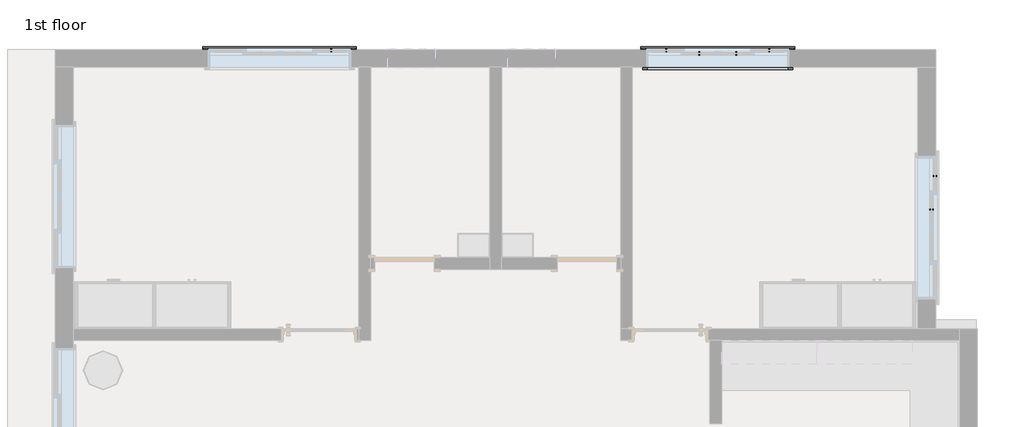
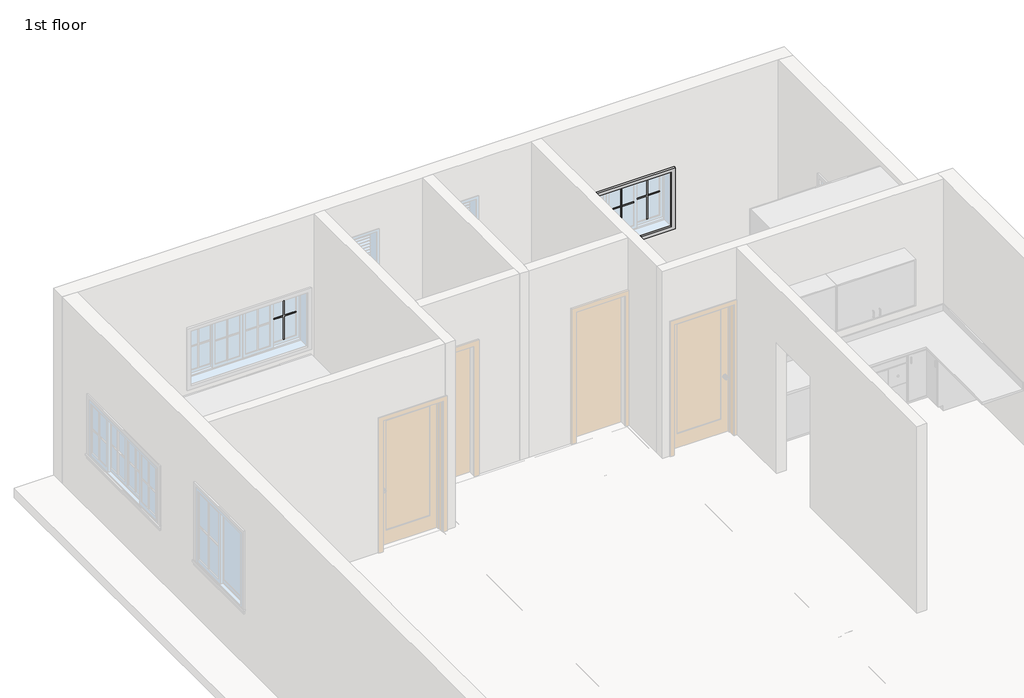
# One storey, part 4 of 4: 10 proxies.
"""IFC4 building model written with IfcOpenShell, lengths in millimetres."""

from ifc_helpers import new_model, si_unit, origin, place, context, project, spatial, transform, mapped, element, save
from components import muntin_pattern_2x2_muntin_pattern_2x2_31a16349, trim_window_exterior_flat_with_sill_3c945769, trim_window_interior_flat_picture_frame_0edfbaa2

model = new_model("IFC4")

# Units and contexts
model_context = context("Model", 3, world=origin())
ifc_project = project(units=[si_unit("LENGTHUNIT", "METRE", prefix="MILLI")], contexts=[model_context])

# Site, building, storey
site = spatial("IfcSite", under=ifc_project)
building = spatial("IfcBuilding", under=site)
storey = spatial("IfcBuildingStorey", under=building, Name="1st floor", Elevation=3810.0)

# Proxies
placement = place(None, origin())
muntin_pattern_2x2_muntin_pattern_2x2_shape = muntin_pattern_2x2_muntin_pattern_2x2_31a16349(model_context)
element("IfcBuildingElementProxy", 1, Name="Muntin Pattern_2x2 : Muntin Pattern_2x2", ObjectType="Muntin Pattern_2x2 : Muntin Pattern_2x2", at=placement, inside=storey, context=model_context, shape_type="MappedRepresentation", body=[
    mapped(muntin_pattern_2x2_muntin_pattern_2x2_shape, transform((-9111.6124084, 10171.2711804, 4806.95), x_axis=(1.0, 0.0, 0.0), y_axis=(0.0, 1.0, 0.0), z_axis=(0.0, 0.0, 1.0))),
])
element("IfcBuildingElementProxy", 2, Name="Muntin Pattern_2x2 : Muntin Pattern_2x2", ObjectType="Muntin Pattern_2x2 : Muntin Pattern_2x2", at=placement, inside=storey, context=model_context, shape_type="MappedRepresentation", body=[
    mapped(muntin_pattern_2x2_muntin_pattern_2x2_shape, transform((-1374.1374084, 8555.1961804, 4806.95), x_axis=(0.0, -1.0, 0.0), y_axis=(1.0, 0.0, 0.0), z_axis=(0.0, 0.0, 1.0))),
])
element("IfcBuildingElementProxy", 3, Name="Muntin Pattern_2x2 : Muntin Pattern_2x2", ObjectType="Muntin Pattern_2x2 : Muntin Pattern_2x2", at=placement, inside=storey, context=model_context, shape_type="MappedRepresentation", body=[
    mapped(muntin_pattern_2x2_muntin_pattern_2x2_shape, transform((-1418.5874084, 8129.7461804, 4806.95), x_axis=(0.0, -1.0, 0.0), y_axis=(1.0, 0.0, 0.0), z_axis=(0.0, 0.0, 1.0))),
])
element("IfcBuildingElementProxy", 4, Name="Muntin Pattern_2x2 : Muntin Pattern_2x2", ObjectType="Muntin Pattern_2x2 : Muntin Pattern_2x2", at=placement, inside=storey, context=model_context, shape_type="MappedRepresentation", body=[
    mapped(muntin_pattern_2x2_muntin_pattern_2x2_shape, transform((-4819.0124084, 10171.2711804, 4806.95), x_axis=(1.0, 0.0, 0.0), y_axis=(0.0, 1.0, 0.0), z_axis=(0.0, 0.0, 1.0))),
])
element("IfcBuildingElementProxy", 5, Name="Muntin Pattern_2x2 : Muntin Pattern_2x2", ObjectType="Muntin Pattern_2x2 : Muntin Pattern_2x2", at=placement, inside=storey, context=model_context, shape_type="MappedRepresentation", body=[
    mapped(muntin_pattern_2x2_muntin_pattern_2x2_shape, transform((-4393.5624084, 10126.8211804, 4806.95), x_axis=(1.0, 0.0, 0.0), y_axis=(0.0, 1.0, 0.0), z_axis=(0.0, 0.0, 1.0))),
])
element("IfcBuildingElementProxy", 6, Name="Muntin Pattern_2x2 : Muntin Pattern_2x2", ObjectType="Muntin Pattern_2x2 : Muntin Pattern_2x2", at=placement, inside=storey, context=model_context, shape_type="MappedRepresentation", body=[
    mapped(muntin_pattern_2x2_muntin_pattern_2x2_shape, transform((-3923.6624084, 10126.8211804, 4806.95), x_axis=(1.0, 0.0, 0.0), y_axis=(0.0, 1.0, 0.0), z_axis=(0.0, 0.0, 1.0))),
])
element("IfcBuildingElementProxy", 7, Name="Muntin Pattern_2x2 : Muntin Pattern_2x2", ObjectType="Muntin Pattern_2x2 : Muntin Pattern_2x2", at=placement, inside=storey, context=model_context, shape_type="MappedRepresentation", body=[
    mapped(muntin_pattern_2x2_muntin_pattern_2x2_shape, transform((-3498.2124084, 10171.2711804, 4806.95), x_axis=(1.0, 0.0, 0.0), y_axis=(0.0, 1.0, 0.0), z_axis=(0.0, 0.0, 1.0))),
])
trim_window_exterior_flat_with_sill_shape = trim_window_exterior_flat_with_sill_3c945769(model_context)
element("IfcBuildingElementProxy", 8, Name="Trim-Window-Exterior-Flat : with Sill", ObjectType="Trim-Window-Exterior-Flat : with Sill", at=placement, inside=storey, context=model_context, shape_type="MappedRepresentation", body=[
    mapped(trim_window_exterior_flat_with_sill_shape, transform((-9772.0124084, 10180.7961804, 5638.8), x_axis=(-1.0, 0.0, 0.0), y_axis=(0.0, 0.0, 1.0), z_axis=(0.0, 1.0, 0.0))),
])
element("IfcBuildingElementProxy", 9, Name="Trim-Window-Exterior-Flat : with Sill", ObjectType="Trim-Window-Exterior-Flat : with Sill", at=placement, inside=storey, context=model_context, shape_type="MappedRepresentation", body=[
    mapped(trim_window_exterior_flat_with_sill_shape, transform((-4158.6124084, 10180.7961804, 5638.8), x_axis=(-1.0, 0.0, 0.0), y_axis=(0.0, 0.0, 1.0), z_axis=(0.0, 1.0, 0.0))),
])
trim_window_interior_flat_picture_frame_shape = trim_window_interior_flat_picture_frame_0edfbaa2(model_context)
element("IfcBuildingElementProxy", 10, Name="Trim-Window-Interior-Flat : Picture Frame", ObjectType="Trim-Window-Interior-Flat : Picture Frame", at=placement, inside=storey, context=model_context, shape_type="MappedRepresentation", body=[
    mapped(trim_window_interior_flat_picture_frame_shape, transform((-4158.6124084, 9952.1961804, 5638.8), x_axis=(1.0, 0.0, 0.0), y_axis=(0.0, 0.0, 1.0), z_axis=(0.0, -1.0, 0.0))),
])

save(model, "model.ifc")

# Revit data of these elements
# Type "Muntin Pattern_2x2 : Muntin Pattern_2x2"
#   Width [instance default] = 4' - 0"
#   Thickness = 0' - 0 1/2"
#   Height [instance default] = 4' - 0"
#   Distance = 0' - 0 3/4"
#   Interior Material [instance default] = none
#   Exterior Material [instance default] = none
#   Default Elevation = 0
# Type "Trim-Window-Exterior-Flat : with Sill"
#   Trim Width = 0' - 2 1/4"
#   Trim Thickness_Picture Frame = 0' - 1 1/4"
#   Trim Thickness_with Sill = 0' - 0 3/4"
#   Sill Thickness = 0' - 1 1/4"
#   Opening Width [instance default] = 2' - 0"
#   Opening Height [instance default] = 3' - 0"
#   Default Elevation = 4' - 0"
#   Sill = yes
#   Picture Frame = no
#   Trim Material [instance default] = none
# Type "Trim-Window-Interior-Flat : Picture Frame"
#   Trim Thickness_Picture Frame = 0' - 1 1/4"
#   Trim Width = 0' - 2 1/4"
#   Trim Thickness_with Sill = 0' - 0 3/4"
#   Sill Thickness = 0' - 1 1/4"
#   Opening Width [instance default] = 2' - 0"
#   Opening Height [instance default] = 3' - 0"
#   Default Elevation = 4' - 0"
#   Sill = no
#   Picture Frame = yes
#   Trim Material [instance default] = none
# Elements 1, 2, 3, 4, 5, 6, 7 (IfcBuildingElementProxy, "Muntin Pattern_2x2 : Muntin Pattern_2x2")
#   Width = 1' - 3"
#   Height = 2' - 6 1/4"
#   Interior Material = Wood - Stained
#   Exterior Material = Clad - White
#   Phase Created = New Construction
#   Materials on its faces: "Clad - White", "Wood - Stained"
# Elements 8, 9 (IfcBuildingElementProxy, "Trim-Window-Exterior-Flat : with Sill")
#   Opening Width = 6' - 0"
#   Opening Height = 3' - 0"
#   Trim Material = Clad - White
#   Phase Created = New Construction
#   Materials on its faces: "Clad - White"
# Element 10 (IfcBuildingElementProxy, "Trim-Window-Interior-Flat : Picture Frame")
#   Opening Width = 6' - 0"
#   Opening Height = 3' - 0"
#   Trim Material = Wood - Stained
#   Phase Created = New Construction
#   Materials on its faces: "Wood - Stained"
# Materials
#   "Clad - White": class "Wood", colour RGB 242 242 238, transparency 0, Cost = 0
#   "Wood - Stained": class "Wood", colour RGB 224 178 126, transparency 0, Cost = 0
